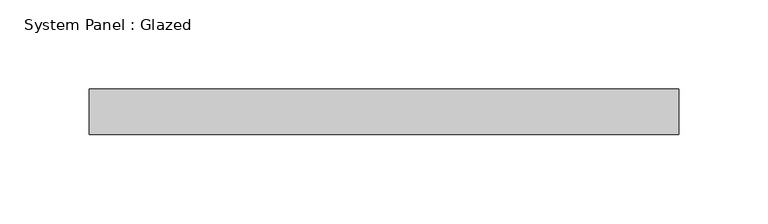
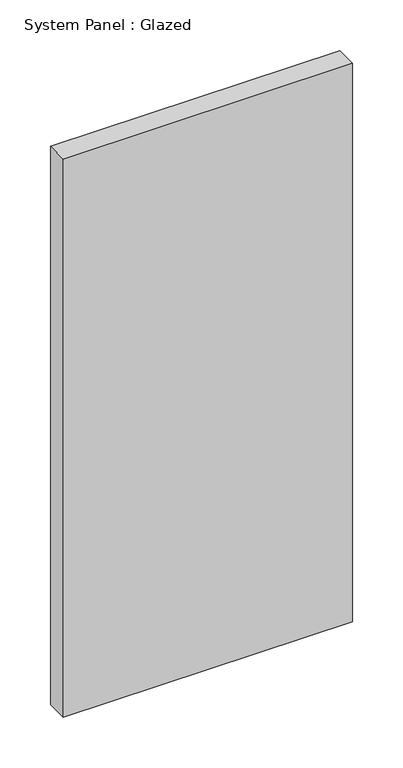
"""IFC4 building model written with IfcOpenShell, lengths in millimetres: plate geometry, System Panel : Glazed."""

from ifc_helpers import new_model, si_unit, origin, origin_with_axes, place, context, project, spatial, polyline, outline, extrude, source, transform, mapped, element, save


def system_panel_glazed_f4e6dc7a(model_context):
    return source(origin(), model_context, "Body", "SweptSolid", [
        extrude(outline(polyline([(165.1, 19.05), (-165.1, 19.05), (-165.1, 44.45), (165.1, 44.45), (165.1, 19.05)])), origin_with_axes(), (0.0, 0.0, 1.0), 673.3295173),
    ])


if __name__ == "__main__":
    model = new_model("IFC4")
    model_context = context("Model", 3, world=origin())
    ifc_project = project(units=[si_unit("LENGTHUNIT", "METRE", prefix="MILLI")], contexts=[model_context])
    site = spatial("IfcSite", under=ifc_project)
    building = spatial("IfcBuilding", under=site)
    placement = place(None, origin())
    system_panel_glazed_shape = system_panel_glazed_f4e6dc7a(model_context)
    element("IfcPlate", 1, ObjectType="System Panel : Glazed", at=placement, inside=building, context=model_context, shape_type="MappedRepresentation", body=[
        mapped(system_panel_glazed_shape, transform((0.0, 0.0, 0.0), x_axis=(1.0, 0.0, 0.0), y_axis=(0.0, 1.0, 0.0), z_axis=(0.0, 0.0, 1.0))),
    ])
    save(model, "model.ifc")

# Revit data of these elements
# Type "System Panel : Glazed"
#   Construction Type Id = "GSP4R"
#   Analytic Construction = "1/8 in Pilkington single glazing"
#   Visual Light Transmittance = 0.9
#   Solar Heat Gain Coefficient = 0.86
#   Heat Transfer Coefficient (U) = 1.18115 BTU/(h·ft²·°F)
#   Define Thermal Properties by = 1
# Element 1 (IfcPlate, "System Panel : Glazed")
#   Materials on its faces: "Glass"
# Materials
#   "Glass": class "Glass", colour RGB 0 128 192, transparency 0.75, Description = "Soda Lime Glass", Cost = 0
